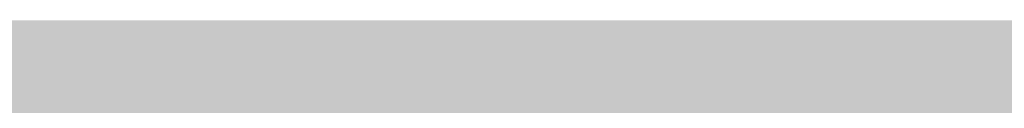
# Model space of a CAD drawing. Units: feet. Extents: x 3168 to 4724, y 827 to 1477.
# Tile 148 of 256: x 3301.14682 to 3301.1638, y 1099.01485 to 1099.01628. Entities that reach past the tile are written whole.
import ezdxf

# ---------------------------------------------------------------- set-up
doc = ezdxf.new("R2010")
doc.units = ezdxf.units.FT
doc.layers.add('A-ELEV', color=7, linetype='Continuous', lineweight=35)
doc.layers.add('A-ELEV-PATT', color=8, linetype='Continuous', lineweight=13)

msp = doc.modelspace()

# ---------------------------------------------------------------- hatches: boundary and pattern name
at = {"layer": 'A-ELEV-PATT'}
h = msp.add_hatch(color=256, dxfattribs=at)
h.dxf.hatch_style = 1
edge = h.paths.add_edge_path()
edge.add_ellipse((3552.905762, 979.220141), major_axis=(36.744924, 0), ratio=0.484848485, start_angle=0, end_angle=360)
edge = h.paths.add_edge_path()
edge.add_ellipse((3559.891637, 929.252282), major_axis=(36.744924, 0), ratio=0.484848485, start_angle=0, end_angle=360)
edge = h.paths.add_edge_path()
edge.add_line((3299.31681, 1198.606081), (3479.916714, 1198.606081))
edge.add_line((3479.916714, 1198.606081), (3479.916714, 1209.86857))
edge.add_spline(control_points=[(3479.916714, 1209.86857), (3464.301157, 1209.86857), (3448.685601, 1209.86857), (3410.949139, 1209.86857), (3388.828234, 1209.86857), (3355.646876, 1209.86857), (3344.586423, 1209.86857), (3327.995745, 1209.86857), (3322.465518, 1209.86857), (3314.170179, 1209.86857), (3311.405066, 1209.86857), (3307.257396, 1209.86857), (3305.874839, 1209.86857), (3303.801005, 1209.86857), (3303.109726, 1209.86857), (3302.072809, 1209.86857), (3301.72717, 1209.86857), (3301.208711, 1209.86857), (3301.035891, 1209.86857), (3300.776662, 1209.86857), (3300.690252, 1209.86857), (3300.560638, 1209.86857), (3300.517433, 1209.86857), (3300.452625, 1209.86857), (3300.431023, 1209.86857), (3300.398619, 1209.86857), (3300.387818, 1209.86857), (3300.366216, 1209.86857), (3300.345676, 1209.86857), (3300.345548, 1209.86857), (3300.345505, 1209.86857), (3300.343304, 1209.86857), (3300.341146, 1209.868571), (3300.337909, 1209.868571), (3300.33683, 1209.868572), (3300.333942, 1209.868573), (3300.332133, 1209.868574), (3300.325515, 1209.868577), (3300.320706, 1209.868581), (3300.310925, 1209.868592), (3300.305952, 1209.868598), (3300.290511, 1209.868623), (3300.280045, 1209.868646), (3300.232425, 1209.868777), (3300.195298, 1209.868954), (3299.951068, 1209.870608), (3299.744824, 1209.874326), (3299.436827, 1209.883257), (3299.334389, 1209.886792), (3299.181079, 1209.89292), (3299.130033, 1209.895099), (3298.652217, 1209.916801), (3298.22946, 1209.945718), (3297.601631, 1210.002367), (3297.393404, 1210.023464), (3297.082652, 1210.058309), (3296.979332, 1210.070458), (3296.292954, 1210.154861), (3295.718148, 1210.243356), (3294.868717, 1210.39885), (3294.5877, 1210.454478), (3294.169341, 1210.543349), (3294.030415, 1210.573878), (3291.707149, 1211.1012), (3289.65359, 1211.813435), (3285.776259, 1213.563988), (3283.95141, 1214.603478), (3280.512159, 1216.98008), (3278.897241, 1218.317592), (3276.379914, 1220.829489), (3275.416042, 1221.917738), (3274.039342, 1223.7077), (3273.581043, 1224.349535), (3273.143228, 1225.016316)], knot_values=[39.119033, 39.119033, 39.119033, 39.119033, 39.286353, 39.286353, 39.523379, 39.523379, 39.641892, 39.641892, 39.701148, 39.701148, 39.730777, 39.730777, 39.745591, 39.745591, 39.752998, 39.752998, 39.756701, 39.756701, 39.758553, 39.758553, 39.759479, 39.759479, 39.759942, 39.759942, 39.760173, 39.760173, 39.760289, 39.760289, 39.760405, 39.760405, 39.760463, 39.760463, 39.763389, 39.763389, 39.764851, 39.764851, 39.767304, 39.767304, 39.773825, 39.773825, 39.78057, 39.78057, 39.79477, 39.79477, 39.845194, 39.845194, 40.126715, 40.126715, 40.267476, 40.267476, 40.337856, 40.337856, 40.927023, 40.927023, 41.221606, 41.221606, 41.368898, 41.368898, 42.202622, 42.202622, 42.619485, 42.619485, 42.827916, 42.827916, 46.118323, 46.118323, 49.408731, 49.408731, 52.699139, 52.699139, 54.927489, 54.927489, 56.104228, 56.104228, 56.104228, 56.104228], weights=[1, 1, 1, 1, 1, 1, 1, 1, 1, 1, 1, 1, 1, 1, 1, 1, 1, 1, 1, 1, 1, 1, 1, 1, 1, 1, 1, 1, 1, 1, 1, 1, 1, 1, 1, 1, 1, 1, 1, 1, 1, 1, 1, 1, 1, 1, 1, 1, 1, 1, 1, 1, 1, 1, 1, 1, 1, 1, 1, 1, 1, 1, 1, 1, 1, 1, 1, 1, 1, 1, 1, 1, 1, 1], degree=3, periodic=0)
edge.add_line((3273.143228, 1225.016316), (3273.143228, 1099.016316))
edge.add_line((3273.143228, 1099.016316), (3299.31681, 1099.016316))
edge.add_line((3299.31681, 1099.016316), (3299.31681, 1198.606081))
edge = h.paths.add_edge_path()
edge.add_line((3304.758443, 1324.15806), (3479.916714, 1324.15806))
edge.add_line((3479.916714, 1324.15806), (3479.916714, 1335.714618))
edge.add_line((3479.916714, 1335.714618), (3269.161628, 1335.714618))
edge.add_spline(control_points=[(3269.161628, 1335.714618), (3264.024231, 1335.714618), (3258.364118, 1328.958189), (3259.264311, 1323.900274)], knot_values=[0, 0, 0, 0, 15.412191, 15.412191, 15.412191, 15.412191], degree=3, periodic=0)
edge.add_line((3259.264311, 1323.900274), (3265.516849, 1288.769135))
edge.add_line((3265.516849, 1288.769135), (3275.265103, 1261.545626))
edge.add_line((3275.265103, 1261.545626), (3304.758443, 1261.545626))
edge.add_line((3304.758443, 1261.545626), (3304.758443, 1324.15806))
h = msp.add_hatch(color=256, dxfattribs=at)
h.dxf.hatch_style = 1
h.paths.add_polyline_path([(3384.525247, 1099.016316), (3335.029168, 1099.016316), (3299.31681, 1099.016316), (3273.143228, 1099.016316), (3217.565364, 1099.016316), (3168.069285, 827.11626), (3335.029168, 827.11626)])

# ---------------------------------------------------------------- linework, layer by layer
at = {"layer": 'A-ELEV'}
msp.add_open_spline([(3808.5202, 1099.016316), (3808.5202, 1141.413235), (3808.5202, 1183.810154), (3808.5202, 1226.635324), (3808.5202, 1227.063576), (3808.5202, 1227.491828), (3811.491871, 1248.994673), (3814.463542, 1270.497518), (3817.46523, 1292.217564), (3817.495247, 1292.434764), (3817.525264, 1292.651964), (3817.572801, 1310.106748), (3817.620339, 1327.561532), (3817.667877, 1345.016316), (3817.667877, 1345.457962), (3817.667877, 1345.899608), (3817.667877, 1346.456047), (3817.667877, 1346.57084), (3817.667877, 1346.752887), (3817.667877, 1346.820142), (3817.667877, 1346.93487), (3817.667877, 1346.982345), (3817.667877, 1347.038587), (3817.667877, 1347.047356), (3817.667877, 1347.073661), (3817.667877, 1347.059303), (3817.667877, 1347.061545), (3817.667876, 1347.062667), (3817.667875, 1347.066031), (3817.667874, 1347.068274), (3817.66787, 1347.075001), (3817.667866, 1347.079486), (3817.667849, 1347.092937), (3817.667833, 1347.101902), (3817.667766, 1347.12879), (3817.667699, 1347.146705), (3817.667432, 1347.200421), (3817.667165, 1347.236192), (3817.6661, 1347.343385), (3817.665038, 1347.414686), (3817.660812, 1347.628095), (3817.656608, 1347.769708), (3817.63997, 1348.192487), (3817.623509, 1348.471586), (3817.559094, 1349.300067), (3817.496121, 1349.840588), (3817.255432, 1351.424156), (3817.026318, 1352.428785), (3816.306871, 1354.888914), (3815.743745, 1356.268727), (3814.463959, 1358.81921), (3813.746413, 1359.990968), (3812.195838, 1362.172343), (3811.362245, 1363.182124), (3809.588836, 1365.069009), (3808.648816, 1365.946105), (3806.654262, 1367.579616), (3805.599702, 1368.336154), (3803.352891, 1369.722327), (3802.160535, 1370.352386), (3799.600813, 1371.453586), (3798.232688, 1371.925481), (3795.280084, 1372.634624), (3793.693148, 1372.872068), (3791.869441, 1372.92648), (3791.740861, 1372.92922), (3791.353371, 1372.934101), (3791.092707, 1372.932901), (3790.304116, 1372.915068), (3789.769543, 1372.884195), (3789.20919, 1372.830236), (3789.190622, 1372.828424), (3789.134892, 1372.822912), (3789.097705, 1372.819137), (3789.048445, 1372.814008), (3789.0364, 1372.812743), (3789.000256, 1372.808918), (3788.976147, 1372.806325), (3788.949405, 1372.803404), (3788.946786, 1372.803118), (3788.942567, 1372.802655), (3788.940967, 1372.80248), (3788.938572, 1372.802217), (3788.937777, 1372.802129), (3788.935391, 1372.801867), (3788.867535, 1372.794402), (3788.756866, 1372.782228), (3788.701532, 1372.776141), (3788.53553, 1372.75788), (3788.424861, 1372.745707), (3788.092856, 1372.709185), (3787.871519, 1372.684837), (3787.207509, 1372.611793), (3786.764835, 1372.563097), (3785.436814, 1372.417009), (3784.551467, 1372.319617), (3781.895425, 1372.027442), (3780.12473, 1371.832658), (3774.812646, 1371.248307), (3771.271256, 1370.858739), (3760.647088, 1369.690037), (3753.56431, 1368.910902), (3732.315973, 1366.573498), (3718.150416, 1365.015228), (3694.006758, 1362.359326), (3684.028657, 1361.261694), (3674.050557, 1360.164062), (3664.600662, 1360.164062), (3655.150767, 1360.164062), (3626.801081, 1360.164062), (3607.901291, 1360.164062), (3551.20192, 1360.164062), (3513.40234, 1360.164062), (3467.725182, 1360.164062), (3459.847604, 1360.164062), (3436.214873, 1360.164062), (3420.459718, 1360.164062), (3373.194255, 1360.164062), (3341.683946, 1360.164062), (3302.848162, 1360.164062), (3295.522686, 1360.164062), (3286.038292, 1360.164062), (3283.879372, 1360.164062), (3277.402613, 1360.164062), (3273.084773, 1360.164062), (3267.732851, 1360.164062), (3266.698768, 1360.164062), (3263.59652, 1360.164062), (3261.528355, 1360.164062), (3259.236943, 1360.164062), (3259.013697, 1360.164062), (3258.343958, 1360.164062), (3257.897466, 1360.164062), (3257.430998, 1360.164062), (3257.411022, 1360.164062), (3257.370573, 1360.164062), (3257.37547, 1360.164062), (3257.374598, 1360.164062), (3257.373937, 1360.164062), (3257.371956, 1360.164062), (3257.370635, 1360.164061), (3257.366673, 1360.16406), (3257.364032, 1360.164059), (3257.356109, 1360.164053), (3257.350828, 1360.164047), (3257.334987, 1360.164023), (3257.32443, 1360.163998), (3257.292769, 1360.163899), (3257.271676, 1360.163799), (3257.208439, 1360.163398), (3257.166337, 1360.162995), (3257.040206, 1360.161388), (3256.956349, 1360.159783), (3256.705504, 1360.153393), (3256.53924, 1360.147036), (3256.04357, 1360.121916), (3255.717296, 1360.097102), (3254.752446, 1360.000481), (3254.127968, 1359.906513), (3252.180067, 1359.525332), (3250.941574, 1359.143991), (3248.670175, 1358.24329), (3247.635739, 1357.723834), (3245.732632, 1356.603471), (3244.863388, 1356.00206), (3243.253108, 1354.742865), (3242.511972, 1354.084731), (3240.751052, 1352.344781), (3239.800961, 1351.229574), (3238.087769, 1348.87244), (3237.324685, 1347.630355), (3235.98251, 1344.971632), (3235.402205, 1343.554907), (3234.591081, 1340.815458), (3234.310882, 1339.54355), (3233.97649, 1336.802561), (3233.922113, 1335.330877), (3234.148916, 1332.591269), (3234.349529, 1331.367201), (3234.719893, 1329.999367), (3234.752423, 1329.883362), (3234.853619, 1329.534797), (3234.925892, 1329.301685), (3235.024836, 1329.002552), (3235.046924, 1328.936928), (3235.077639, 1328.847239), (3235.085924, 1328.823198), (3235.110939, 1328.751064), (3235.127828, 1328.702962), (3235.147992, 1328.646242), (3235.151059, 1328.637632), (3235.156096, 1328.623526), (3235.158061, 1328.61803), (3235.160209, 1328.61203), (3235.165612, 1328.596943), (3235.180099, 1328.556486), (3235.190263, 1328.528101), (3235.220756, 1328.442946), (3235.241084, 1328.386176), (3235.302069, 1328.215865), (3235.342726, 1328.102325), (3235.464696, 1327.761704), (3235.54601, 1327.534623), (3235.78995, 1326.853381), (3235.952577, 1326.39922), (3236.440459, 1325.036736), (3236.765713, 1324.128414), (3237.741475, 1321.403446), (3238.391983, 1319.586801), (3240.343508, 1314.136866), (3241.644525, 1310.503576), (3245.547574, 1299.603706), (3248.149607, 1292.337126), (3255.955706, 1270.537385), (3261.159772, 1256.004225), (3267.387618, 1238.612001), (3268.411397, 1235.752937), (3269.510378, 1232.683864), (3269.585579, 1232.473854), (3269.706612, 1232.135851), (3269.752444, 1232.007857), (3269.827329, 1231.79873), (3269.856382, 1231.717595), (3269.906325, 1231.578122), (3269.927215, 1231.519782), (3269.972468, 1231.393406), (3269.996831, 1231.325368), (3270.026503, 1231.242506), (3270.031811, 1231.227681), (3270.040282, 1231.204024), (3270.039224, 1231.206979), (3270.039359, 1231.206601), (3270.039427, 1231.206412), (3270.03963, 1231.205846), (3270.039765, 1231.205468), (3270.040171, 1231.204335), (3270.040442, 1231.203579), (3270.041254, 1231.201313), (3270.041796, 1231.199802), (3270.04342, 1231.195269), (3270.044504, 1231.192248), (3270.047756, 1231.183185), (3270.049926, 1231.177145), (3270.056442, 1231.159028), (3270.060793, 1231.146957), (3270.073867, 1231.110761), (3270.082613, 1231.086656), (3270.108936, 1231.014413), (3270.1266, 1230.96635), (3270.179934, 1230.822457), (3270.215947, 1230.726923), (3270.325323, 1230.441508), (3270.400026, 1230.252811), (3270.629249, 1229.691444), (3270.788883, 1229.323501), (3271.286488, 1228.238319), (3271.6431, 1227.539755), (3272.775859, 1225.515277), (3273.614169, 1224.260502), (3275.416042, 1221.917738), (3276.379914, 1220.829489), (3278.897241, 1218.317592), (3280.512159, 1216.98008), (3283.95141, 1214.603478), (3285.776259, 1213.563988), (3289.65359, 1211.813435), (3291.707149, 1211.1012), (3294.030415, 1210.573878), (3294.169341, 1210.543349), (3294.5877, 1210.454478), (3294.868717, 1210.39885), (3295.718148, 1210.243356), (3296.292954, 1210.154861), (3296.979332, 1210.070458), (3297.082652, 1210.058309), (3297.393404, 1210.023464), (3297.601631, 1210.002367), (3298.22946, 1209.945718), (3298.652217, 1209.916801), (3299.130033, 1209.895099), (3299.181079, 1209.89292), (3299.334389, 1209.886792), (3299.436827, 1209.883257), (3299.744824, 1209.874326), (3299.951068, 1209.870608), (3300.195298, 1209.868954), (3300.232425, 1209.868777), (3300.280045, 1209.868646), (3300.290511, 1209.868623), (3300.305952, 1209.868598), (3300.310925, 1209.868592), (3300.320706, 1209.868581), (3300.325515, 1209.868577), (3300.332133, 1209.868574), (3300.333942, 1209.868573), (3300.33683, 1209.868572), (3300.337909, 1209.868571), (3300.341146, 1209.868571), (3300.343304, 1209.86857), (3300.345505, 1209.86857), (3300.345548, 1209.86857), (3300.345676, 1209.86857), (3300.366216, 1209.86857), (3300.387818, 1209.86857), (3300.398619, 1209.86857), (3300.431023, 1209.86857), (3300.452625, 1209.86857), (3300.517433, 1209.86857), (3300.560638, 1209.86857), (3300.690252, 1209.86857), (3300.776662, 1209.86857), (3301.035891, 1209.86857), (3301.208711, 1209.86857), (3301.72717, 1209.86857), (3302.072809, 1209.86857), (3303.109726, 1209.86857), (3303.801005, 1209.86857), (3305.874839, 1209.86857), (3307.257396, 1209.86857), (3311.405066, 1209.86857), (3314.170179, 1209.86857), (3322.465518, 1209.86857), (3327.995745, 1209.86857), (3344.586423, 1209.86857), (3355.646876, 1209.86857), (3388.828234, 1209.86857), (3410.949139, 1209.86857), (3477.311855, 1209.86857), (3521.553665, 1209.86857), (3566.836184, 1209.86857), (3567.876892, 1209.86857), (3570.999017, 1209.86857), (3573.080433, 1209.86857), (3575.781396, 1209.86857), (3576.400943, 1209.86857), (3577.295821, 1209.86857), (3577.571152, 1209.86857), (3578.397146, 1209.86857), (3578.947808, 1209.86857), (3579.756491, 1209.86857), (3580.014511, 1209.86857), (3580.342737, 1209.86857), (3580.326865, 1209.86857), (3580.32717, 1209.86857), (3580.327323, 1209.86857), (3580.327781, 1209.86857), (3580.328086, 1209.86857), (3580.329002, 1209.86857), (3580.329613, 1209.86857), (3580.331445, 1209.86857), (3580.332667, 1209.86857), (3580.336332, 1209.868569), (3580.338775, 1209.868567), (3580.346107, 1209.868563), (3580.350995, 1209.868558), (3580.365663, 1209.86854), (3580.375445, 1209.868522), (3580.404801, 1209.868449), (3580.424386, 1209.868376), (3580.483183, 1209.868085), (3580.522437, 1209.867793), (3580.640361, 1209.866624), (3580.719195, 1209.865454), (3580.956315, 1209.860766), (3581.115222, 1209.85607), (3581.594164, 1209.83723), (3581.916419, 1209.818331), (3582.889947, 1209.742428), (3583.547986, 1209.666169), (3585.531827, 1209.360617), (3586.867216, 1209.053886), (3589.471545, 1208.252472), (3590.740241, 1207.757852), (3591.995451, 1207.158802), (3592.057809, 1207.12874), (3592.244242, 1207.037954), (3592.367676, 1206.976632), (3592.73528, 1206.790359), (3592.976752, 1206.663101), (3593.244539, 1206.516441), (3593.274731, 1206.499825), (3593.365115, 1206.449839), (3593.425113, 1206.416333), (3593.604314, 1206.315285), (3593.722725, 1206.247211), (3593.857212, 1206.168398), (3593.874362, 1206.158319), (3593.925741, 1206.128041), (3593.959899, 1206.107798), (3594.062086, 1206.046899), (3594.129827, 1206.006074), (3594.208436, 1205.958171), (3594.219683, 1205.951304), (3594.253391, 1205.930686), (3594.275819, 1205.916917), (3594.342972, 1205.875536), (3594.387563, 1205.847853), (3594.433616, 1205.81905), (3594.435256, 1205.818024), (3594.440175, 1205.814946), (3594.443453, 1205.812894), (3594.447123, 1205.810594), (3594.447516, 1205.810348), (3594.448695, 1205.80961), (3594.449481, 1205.809117), (3594.450366, 1205.808562), (3594.450466, 1205.8085), (3594.4506, 1205.808415), (3594.467399, 1205.797887), (3594.493269, 1205.781674), (3594.506204, 1205.773568), (3594.545008, 1205.749248), (3594.570878, 1205.733035), (3594.648487, 1205.684396), (3594.700226, 1205.651969), (3594.855444, 1205.554691), (3594.958922, 1205.489839), (3595.269357, 1205.295282), (3595.476314, 1205.165577), (3596.097185, 1204.776463), (3596.511099, 1204.517054), (3597.752841, 1203.738826), (3598.580669, 1203.220007), (3601.064152, 1201.663551), (3602.719807, 1200.625914), (3607.686774, 1197.513002), (3610.998085, 1195.437727), (3620.932018, 1189.211903), (3627.55464, 1185.061354), (3647.422507, 1172.609707), (3660.667751, 1164.308608), (3700.403484, 1139.405313), (3726.893973, 1122.803116), (3757.205715, 1103.806052), (3761.02697, 1101.411184), (3764.848224, 1099.016316), (3745.328271, 1099.016316), (3725.808319, 1099.016316), (3706.288366, 1099.016316), (3706.288366, 1108.453237), (3706.288366, 1117.890158), (3706.288366, 1127.327079), (3710.750754, 1127.327079), (3715.213143, 1127.327079), (3719.675531, 1127.327079)], degree=3, knots=[0, 0, 0, 0, 0.982037, 0.982037, 0.991957, 0.991957, 0.991957, 1.966522, 1.966522, 1.976367, 1.976367, 1.976367, 2.976367, 2.976367, 2.976367, 3.00169, 3.00169, 3.008272, 3.008272, 3.012129, 3.012129, 3.014851, 3.014851, 3.015353, 3.015353, 3.016359, 3.016359, 3.017365, 3.017365, 3.019376, 3.019376, 3.023398, 3.023398, 3.031442, 3.031442, 3.047531, 3.047531, 3.079708, 3.079708, 3.144063, 3.144063, 3.272772, 3.272772, 3.53019, 3.53019, 4.045026, 4.045026, 5.074698, 5.074698, 6.700878, 6.700878, 8.327058, 8.327058, 9.953238, 9.953238, 11.579418, 11.579418, 13.205598, 13.205598, 14.831778, 14.831778, 16.457958, 16.457958, 18.084138, 18.084138, 18.206872, 18.206872, 18.45234, 18.45234, 18.943275, 18.943275, 18.960093, 18.960093, 18.993729, 18.993729, 19.00461, 19.00461, 19.026374, 19.026374, 19.028737, 19.028737, 19.03018, 19.03018, 19.030897, 19.030897, 19.032332, 19.032332, 19.033766, 19.033766, 19.036636, 19.036636, 19.042374, 19.042374, 19.053851, 19.053851, 19.076805, 19.076805, 19.122714, 19.122714, 19.21453, 19.21453, 19.398163, 19.398163, 19.765429, 19.765429, 20.024128, 20.024128, 20.024128, 20.092031, 20.092031, 20.227836, 20.227836, 20.499446, 20.499446, 20.556051, 20.556051, 20.66926, 20.66926, 20.895678, 20.895678, 20.948316, 20.948316, 20.963829, 20.963829, 20.994855, 20.994855, 21.002285, 21.002285, 21.017146, 21.017146, 21.01875, 21.01875, 21.021959, 21.021959, 21.022102, 21.022102, 21.022249, 21.022249, 21.022708, 21.022708, 21.023627, 21.023627, 21.025464, 21.025464, 21.029138, 21.029138, 21.036486, 21.036486, 21.051183, 21.051183, 21.080575, 21.080575, 21.139361, 21.139361, 21.256932, 21.256932, 21.492073, 21.492073, 21.962356, 21.962356, 23.01002, 23.01002, 24.057684, 24.057684, 25.105348, 25.105348, 26.153011, 26.153011, 27.776787, 27.776787, 29.400562, 29.400562, 31.024337, 31.024337, 32.278801, 32.278801, 33.533265, 33.533265, 34.467568, 34.467568, 34.553971, 34.553971, 34.726776, 34.726776, 34.775309, 34.775309, 34.793079, 34.793079, 34.82862, 34.82862, 34.834979, 34.834979, 34.839039, 34.839039, 34.839411, 34.839411, 34.840285, 34.840285, 34.842034, 34.842034, 34.845531, 34.845531, 34.852525, 34.852525, 34.866512, 34.866512, 34.894488, 34.894488, 34.950439, 34.950439, 35.062342, 35.062342, 35.286147, 35.286147, 35.733758, 35.733758, 35.821815, 35.821815, 35.828283, 35.828283, 35.832225, 35.832225, 35.834724, 35.834724, 35.836521, 35.836521, 35.838617, 35.838617, 35.839073, 35.839073, 35.839345, 35.839345, 35.839617, 35.839617, 35.840161, 35.840161, 35.841249, 35.841249, 35.843425, 35.843425, 35.847778, 35.847778, 35.856482, 35.856482, 35.873891, 35.873891, 35.908709, 35.908709, 35.978345, 35.978345, 36.117617, 36.117617, 36.396161, 36.396161, 36.953248, 36.953248, 38.067423, 38.067423, 40.295772, 40.295772, 42.524122, 42.524122, 45.81453, 45.81453, 49.104937, 49.104937, 52.395345, 52.395345, 52.603776, 52.603776, 53.020639, 53.020639, 53.854363, 53.854363, 54.001655, 54.001655, 54.296238, 54.296238, 54.885405, 54.885405, 54.955785, 54.955785, 55.096546, 55.096546, 55.378067, 55.378067, 55.42849, 55.42849, 55.442691, 55.442691, 55.449436, 55.449436, 55.455957, 55.455957, 55.458409, 55.458409, 55.459872, 55.459872, 55.462798, 55.462798, 55.462856, 55.462856, 55.462972, 55.462972, 55.463088, 55.463088, 55.463319, 55.463319, 55.463782, 55.463782, 55.464708, 55.464708, 55.46656, 55.46656, 55.470263, 55.470263, 55.47767, 55.47767, 55.492484, 55.492484, 55.522112, 55.522112, 55.581369, 55.581369, 55.699882, 55.699882, 55.936907, 55.936907, 56.410959, 56.410959, 56.42211, 56.42211, 56.444413, 56.444413, 56.451051, 56.451051, 56.454001, 56.454001, 56.459901, 56.459901, 56.462666, 56.462666, 56.463418, 56.463418, 56.464171, 56.464171, 56.465675, 56.465675, 56.468684, 56.468684, 56.474702, 56.474702, 56.486738, 56.486738, 56.51081, 56.51081, 56.558955, 56.558955, 56.655243, 56.655243, 56.847821, 56.847821, 57.232975, 57.232975, 58.003284, 58.003284, 59.543901, 59.543901, 62.625137, 62.625137, 68.787607, 68.787607, 74.950078, 74.950078, 75.27336, 75.27336, 75.919923, 75.919923, 77.213051, 77.213051, 77.377769, 77.377769, 77.707206, 77.707206, 78.366079, 78.366079, 78.462532, 78.462532, 78.655436, 78.655436, 79.041245, 79.041245, 79.105735, 79.105735, 79.234714, 79.234714, 79.492672, 79.492672, 79.502197, 79.502197, 79.521249, 79.521249, 79.523534, 79.523534, 79.528103, 79.528103, 79.528682, 79.528682, 79.528885, 79.528885, 79.529089, 79.529089, 79.529495, 79.529495, 79.530308, 79.530308, 79.531935, 79.531935, 79.535187, 79.535187, 79.541693, 79.541693, 79.554704, 79.554704, 79.580725, 79.580725, 79.632769, 79.632769, 79.736856, 79.736856, 79.94503, 79.94503, 80.361377, 80.361377, 80.421435, 80.421435, 80.421435, 81.421435, 81.421435, 81.421435, 82.421435, 82.421435, 82.421435, 83.421435, 83.421435, 83.421435, 83.421435], dxfattribs=at)

doc.saveas('drawing.dxf')
